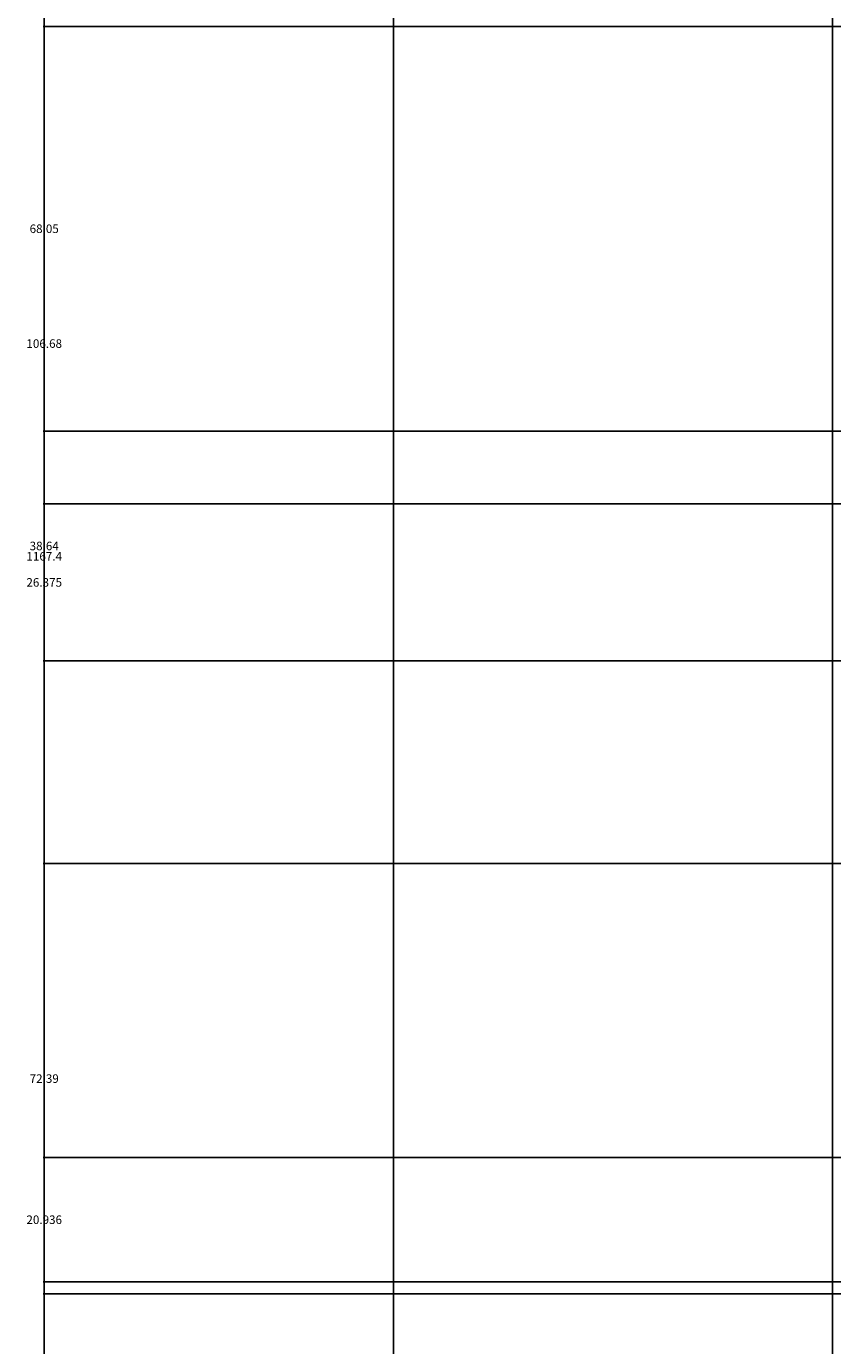
# Model space of a CAD drawing. Units: inches. Extents: x 241 to 943, y 109 to 1396.
# Tile 9 of 34: x 241 to 377, y 620 to 842. Entities that reach past the tile are written whole.
import ezdxf

# ---------------------------------------------------------------- set-up
doc = ezdxf.new("R2010")
doc.units = ezdxf.units.IN
doc.header["$MEASUREMENT"] = 0
doc.layers.add('A-ANNO-DIMS', color=2, linetype='Continuous', lineweight=18)
doc.styles.get("Standard").update_dxf_attribs({"font": 'arial.ttf'})
doc.dimstyles.get("Standard").update_dxf_attribs({"dimtxt": 1.4375, "dimasz": 0.18, "dimexe": 0.18, "dimexo": 0.0625, "dimgap": 0.09, "dimtad": 0, "dimtih": 1, "dimtoh": 1, "dimdec": 4, "dimzin": 0, "dimdsep": 46, "dimlunit": 4, "dimtxsty": 'Standard', "dimcen": 0.09, "dimadec": 0, "dimazin": 0, "dimtfac": 1, "dimtdec": 4, "dimtofl": 0, "dimtmove": 0, "dimatfit": 3, "dimfxl": 1, "dimtolj": 1, "dimtzin": 0, "dimarcsym": 0})

# ---------------------------------------------------------------- blocks, each defined once
blk = doc.blocks.new('*D5')
at = {"layer": 'A-ANNO-DIMS', "color": 0, "lineweight": -2, "transparency": 16777216}
for p, q in [((303.24, 177.8), (303.24, 1395.05)), ((303.42, 1394.87), (338.18, 1394.87)), ((376.86, 1394.87), (342.09, 1394.87)), ((377.04, 177.76), (377.04, 1395.05))]:
    blk.add_line(p, q, dxfattribs=at)
at = {"layer": 'A-ANNO-DIMS', "color": 0, "transparency": 16777216}
for points in [[(303.42, 1394.9), (303.42, 1394.84), (303.24, 1394.87)], [(376.86, 1394.9), (376.86, 1394.84), (377.04, 1394.87)]]:
    blk.add_solid(points, dxfattribs=at)
at = {"layer": 'Defpoints', "color": 0, "transparency": 16777216}
for p in [(377.04, 1394.87), (303.24, 177.74), (377.04, 177.7)]:
    blk.add_point(p, dxfattribs=at)
at = {"layer": 'A-ANNO-DIMS', "color": 0, "transparency": 16777216, "insert": (340.14, 1394.87), "char_height": 1.438, "attachment_point": 5}
blk.add_mtext('\\A1;73.8', dxfattribs=at)
blk = doc.blocks.new('*D7')
at = {"layer": 'A-ANNO-DIMS', "color": 0, "lineweight": -2, "transparency": 16777216}
for p, q in [((508.24, 1336.12), (244.31, 1336.12)), ((244.49, 1335.94), (244.49, 753.25)), ((244.49, 168.92), (244.49, 751.6)), ((303.17, 168.74), (244.31, 168.74))]:
    blk.add_line(p, q, dxfattribs=at)
at = {"layer": 'A-ANNO-DIMS', "color": 0, "transparency": 16777216}
for points in [[(244.46, 1335.94), (244.52, 1335.94), (244.49, 1336.12)], [(244.46, 168.92), (244.52, 168.92), (244.49, 168.74)]]:
    blk.add_solid(points, dxfattribs=at)
at = {"layer": 'Defpoints', "color": 0, "transparency": 16777216}
for p in [(244.49, 1336.12), (508.31, 1336.12), (303.24, 168.74)]:
    blk.add_point(p, dxfattribs=at)
at = {"layer": 'A-ANNO-DIMS', "color": 0, "transparency": 16777216, "insert": (244.49, 752.43), "char_height": 1.438, "attachment_point": 5}
blk.add_mtext('\\A1;1167.4', dxfattribs=at)
blk = doc.blocks.new('*D8')
at = {"layer": 'A-ANNO-DIMS', "color": 0, "lineweight": -2, "transparency": 16777216}
for p, q in [((377.04, 396.94), (377.04, 1395.05)), ((377.22, 1394.87), (380.96, 1394.87)), ((390.71, 1394.87), (386.97, 1394.87)), ((390.89, 384.24), (390.89, 1395.05))]:
    blk.add_line(p, q, dxfattribs=at)
at = {"layer": 'A-ANNO-DIMS', "color": 0, "transparency": 16777216}
for points in [[(377.22, 1394.9), (377.22, 1394.84), (377.04, 1394.87)], [(390.71, 1394.9), (390.71, 1394.84), (390.89, 1394.87)]]:
    blk.add_solid(points, dxfattribs=at)
at = {"layer": 'Defpoints', "color": 0, "transparency": 16777216}
for p in [(390.89, 1394.87), (377.04, 396.88), (390.89, 384.18)]:
    blk.add_point(p, dxfattribs=at)
at = {"layer": 'A-ANNO-DIMS', "color": 0, "transparency": 16777216, "insert": (383.97, 1394.87), "char_height": 1.438, "attachment_point": 5}
blk.add_mtext('\\A1;13.856', dxfattribs=at)
blk = doc.blocks.new('*D21')
at = {"layer": 'A-ANNO-DIMS', "color": 0, "lineweight": -2, "transparency": 16777216}
for p, q in [((376.98, 734.85), (244.31, 734.85)), ((244.49, 734.67), (244.49, 568.67)), ((244.49, 401.01), (244.49, 567.02)), ((376.98, 400.83), (244.31, 400.83))]:
    blk.add_line(p, q, dxfattribs=at)
at = {"layer": 'A-ANNO-DIMS', "color": 0, "transparency": 16777216}
for points in [[(244.46, 734.67), (244.52, 734.67), (244.49, 734.85)], [(244.46, 401.01), (244.52, 401.01), (244.49, 400.83)]]:
    blk.add_solid(points, dxfattribs=at)
at = {"layer": 'Defpoints', "color": 0, "transparency": 16777216}
for p in [(244.49, 734.85), (377.04, 734.85), (377.04, 400.83)]:
    blk.add_point(p, dxfattribs=at)
at = {"layer": 'A-ANNO-DIMS', "color": 0, "transparency": 16777216, "insert": (244.49, 567.84), "char_height": 1.438, "attachment_point": 5}
blk.add_mtext('\\A1;334', dxfattribs=at)
blk = doc.blocks.new('*D22')
at = {"layer": 'A-ANNO-DIMS', "color": 0, "lineweight": -2, "transparency": 16777216}
for p, q in [((376.98, 841.54), (244.31, 841.54)), ((244.49, 841.36), (244.49, 789.02)), ((244.49, 735.03), (244.49, 787.37)), ((376.98, 734.85), (244.31, 734.85))]:
    blk.add_line(p, q, dxfattribs=at)
at = {"layer": 'A-ANNO-DIMS', "color": 0, "transparency": 16777216}
for points in [[(244.46, 841.36), (244.52, 841.36), (244.49, 841.54)], [(244.46, 735.03), (244.52, 735.03), (244.49, 734.85)]]:
    blk.add_solid(points, dxfattribs=at)
at = {"layer": 'Defpoints', "color": 0, "transparency": 16777216}
for p in [(244.49, 841.54), (377.04, 841.54), (377.04, 734.85)]:
    blk.add_point(p, dxfattribs=at)
at = {"layer": 'A-ANNO-DIMS', "color": 0, "transparency": 16777216, "insert": (244.49, 788.2), "char_height": 1.438, "attachment_point": 5}
blk.add_mtext('\\A1;106.68', dxfattribs=at)
blk = doc.blocks.new('*D33')
at = {"layer": 'A-ANNO-DIMS', "color": 0, "lineweight": -2, "transparency": 16777216}
for p, q in [((424.05, 628.4), (244.31, 628.4)), ((244.49, 628.22), (244.49, 599.44)), ((244.49, 569.01), (244.49, 597.79)), ((424.05, 568.83), (244.31, 568.83))]:
    blk.add_line(p, q, dxfattribs=at)
at = {"layer": 'A-ANNO-DIMS', "color": 0, "transparency": 16777216}
for points in [[(244.46, 628.22), (244.52, 628.22), (244.49, 628.4)], [(244.46, 569.01), (244.52, 569.01), (244.49, 568.83)]]:
    blk.add_solid(points, dxfattribs=at)
at = {"layer": 'Defpoints', "color": 0, "transparency": 16777216}
for p in [(244.49, 628.4), (424.11, 628.4), (424.11, 568.83)]:
    blk.add_point(p, dxfattribs=at)
at = {"layer": 'A-ANNO-DIMS', "color": 0, "transparency": 16777216, "insert": (244.49, 598.62), "char_height": 1.438, "attachment_point": 5}
blk.add_mtext('\\A1;59.57', dxfattribs=at)
blk = doc.blocks.new('*D34')
at = {"layer": 'A-ANNO-DIMS', "color": 0, "lineweight": -2, "transparency": 16777216}
for p, q in [((424.05, 700.79), (244.31, 700.79)), ((244.49, 700.61), (244.49, 665.42)), ((244.49, 628.58), (244.49, 663.77)), ((424.05, 628.4), (244.31, 628.4))]:
    blk.add_line(p, q, dxfattribs=at)
at = {"layer": 'A-ANNO-DIMS', "color": 0, "transparency": 16777216}
for points in [[(244.46, 700.61), (244.52, 700.61), (244.49, 700.79)], [(244.46, 628.58), (244.52, 628.58), (244.49, 628.4)]]:
    blk.add_solid(points, dxfattribs=at)
at = {"layer": 'Defpoints', "color": 0, "transparency": 16777216}
for p in [(244.49, 700.79), (424.11, 700.79), (424.11, 628.4)]:
    blk.add_point(p, dxfattribs=at)
at = {"layer": 'A-ANNO-DIMS', "color": 0, "transparency": 16777216, "insert": (244.49, 664.6), "char_height": 1.438, "attachment_point": 5}
blk.add_mtext('\\A1;72.39', dxfattribs=at)
blk = doc.blocks.new('*D35')
at = {"layer": 'A-ANNO-DIMS', "color": 0, "lineweight": -2, "transparency": 16777216}
for p, q in [((388.98, 773.49), (244.31, 773.49)), ((244.49, 773.31), (244.49, 755)), ((244.49, 735.03), (244.49, 753.35)), ((388.98, 734.85), (244.31, 734.85))]:
    blk.add_line(p, q, dxfattribs=at)
at = {"layer": 'A-ANNO-DIMS', "color": 0, "transparency": 16777216}
for points in [[(244.46, 773.31), (244.52, 773.31), (244.49, 773.49)], [(244.46, 735.03), (244.52, 735.03), (244.49, 734.85)]]:
    blk.add_solid(points, dxfattribs=at)
at = {"layer": 'Defpoints', "color": 0, "transparency": 16777216}
for p in [(244.49, 773.49), (389.04, 773.49), (389.04, 734.85)]:
    blk.add_point(p, dxfattribs=at)
at = {"layer": 'A-ANNO-DIMS', "color": 0, "transparency": 16777216, "insert": (244.49, 754.17), "char_height": 1.438, "attachment_point": 5}
blk.add_mtext('\\A1;38.64', dxfattribs=at)
blk = doc.blocks.new('*D36')
at = {"layer": 'A-ANNO-DIMS', "color": 0, "lineweight": -2, "transparency": 16777216}
for p, q in [((396.25, 841.54), (244.31, 841.54)), ((244.49, 841.36), (244.49, 808.34)), ((244.49, 773.67), (244.49, 806.69)), ((396.25, 773.49), (244.31, 773.49))]:
    blk.add_line(p, q, dxfattribs=at)
at = {"layer": 'A-ANNO-DIMS', "color": 0, "transparency": 16777216}
for points in [[(244.46, 841.36), (244.52, 841.36), (244.49, 841.54)], [(244.46, 773.67), (244.52, 773.67), (244.49, 773.49)]]:
    blk.add_solid(points, dxfattribs=at)
at = {"layer": 'Defpoints', "color": 0, "transparency": 16777216}
for p in [(244.49, 841.54), (396.31, 841.54), (396.31, 773.49)]:
    blk.add_point(p, dxfattribs=at)
at = {"layer": 'A-ANNO-DIMS', "color": 0, "transparency": 16777216, "insert": (244.49, 807.51), "char_height": 1.438, "attachment_point": 5}
blk.add_mtext('\\A1;68.05', dxfattribs=at)
blk = doc.blocks.new('*D61')
at = {"layer": 'A-ANNO-DIMS', "color": 0, "lineweight": -2, "transparency": 16777216}
for p, q in [((377.04, 400.89), (377.04, 1395.05)), ((377.22, 1394.87), (398.03, 1394.87)), ((423.93, 1394.87), (403.12, 1394.87)), ((424.11, 568.89), (424.11, 1395.05))]:
    blk.add_line(p, q, dxfattribs=at)
at = {"layer": 'A-ANNO-DIMS', "color": 0, "transparency": 16777216}
for points in [[(377.22, 1394.9), (377.22, 1394.84), (377.04, 1394.87)], [(423.93, 1394.9), (423.93, 1394.84), (424.11, 1394.87)]]:
    blk.add_solid(points, dxfattribs=at)
at = {"layer": 'Defpoints', "color": 0, "transparency": 16777216}
for p in [(424.11, 1394.87), (424.11, 568.83), (377.04, 400.83)]:
    blk.add_point(p, dxfattribs=at)
at = {"layer": 'A-ANNO-DIMS', "color": 0, "transparency": 16777216, "insert": (400.57, 1394.87), "char_height": 1.438, "attachment_point": 5}
blk.add_mtext('\\A1;47.07', dxfattribs=at)
blk = doc.blocks.new('*D91')
at = {"layer": 'A-ANNO-DIMS', "color": 0, "lineweight": -2, "transparency": 16777216}
for p, q in [((377.04, 1070.79), (377.04, 109.81)), ((389.04, 1070.79), (389.04, 109.81)), ((377.22, 109.99), (380.04, 109.99)), ((388.86, 109.99), (386.04, 109.99))]:
    blk.add_line(p, q, dxfattribs=at)
at = {"layer": 'A-ANNO-DIMS', "color": 0, "transparency": 16777216}
for points in [[(377.22, 110.02), (377.22, 109.96), (377.04, 109.99)], [(388.86, 110.02), (388.86, 109.96), (389.04, 109.99)]]:
    blk.add_solid(points, dxfattribs=at)
at = {"layer": 'Defpoints', "color": 0, "transparency": 16777216}
for p in [(377.04, 1070.85), (389.04, 1070.85), (389.04, 109.99)]:
    blk.add_point(p, dxfattribs=at)
at = {"layer": 'A-ANNO-DIMS', "color": 0, "transparency": 16777216, "insert": (383.04, 109.99), "char_height": 1.438, "attachment_point": 5}
blk.add_mtext('\\A1;12.004', dxfattribs=at)
blk = doc.blocks.new('*D131')
at = {"layer": 'A-ANNO-DIMS', "color": 0, "lineweight": -2, "transparency": 16777216}
for p, q in [((446.37, 651.34), (244.31, 651.34)), ((244.49, 651.16), (244.49, 641.69)), ((244.49, 630.58), (244.49, 640.04)), ((446.37, 630.4), (244.31, 630.4))]:
    blk.add_line(p, q, dxfattribs=at)
at = {"layer": 'A-ANNO-DIMS', "color": 0, "transparency": 16777216}
for points in [[(244.46, 651.16), (244.52, 651.16), (244.49, 651.34)], [(244.46, 630.58), (244.52, 630.58), (244.49, 630.4)]]:
    blk.add_solid(points, dxfattribs=at)
at = {"layer": 'Defpoints', "color": 0, "transparency": 16777216}
for p in [(244.49, 651.34), (446.43, 651.34), (446.43, 630.4)]:
    blk.add_point(p, dxfattribs=at)
at = {"layer": 'A-ANNO-DIMS', "color": 0, "transparency": 16777216, "insert": (244.49, 640.87), "char_height": 1.438, "attachment_point": 5}
blk.add_mtext('\\A1;20.936', dxfattribs=at)
blk = doc.blocks.new('*D149')
at = {"layer": 'A-ANNO-DIMS', "color": 0, "lineweight": -2, "transparency": 16777216}
for p, q in [((413.06, 761.23), (244.31, 761.23)), ((244.49, 761.05), (244.49, 748.87)), ((244.49, 735.03), (244.49, 747.22)), ((413.06, 734.85), (244.31, 734.85))]:
    blk.add_line(p, q, dxfattribs=at)
at = {"layer": 'A-ANNO-DIMS', "color": 0, "transparency": 16777216}
for points in [[(244.46, 761.05), (244.52, 761.05), (244.49, 761.23)], [(244.46, 735.03), (244.52, 735.03), (244.49, 734.85)]]:
    blk.add_solid(points, dxfattribs=at)
at = {"layer": 'Defpoints', "color": 0, "transparency": 16777216}
for p in [(244.49, 761.23), (413.12, 761.23), (413.12, 734.85)]:
    blk.add_point(p, dxfattribs=at)
at = {"layer": 'A-ANNO-DIMS', "color": 0, "transparency": 16777216, "insert": (244.49, 748.04), "char_height": 1.438, "attachment_point": 5}
blk.add_mtext('\\A1;26.375', dxfattribs=at)

msp = doc.modelspace()

# ---------------------------------------------------------------- dimensions: what is measured, and where the dimension line sits
at = {"layer": 'A-ANNO-DIMS'}
for base, p1, p2, override, picture, middle in [((377.0391, 1394.8654), (303.2358, 177.7407), (377.0391, 177.6977), {"dimdec": 1, "dimlfac": 1, "dimrnd": 0, "dimzin": 0, "dimdsep": 46, "dimlunit": 2}, '*D5', (340.1375, 1394.8654)), ((390.895, 1394.8654), (377.0391, 396.8782), (390.895, 384.1784), {"dimdec": 3, "dimlfac": 1, "dimrnd": 0, "dimzin": 0, "dimdsep": 46, "dimlunit": 2}, '*D8', (383.9671, 1394.8654)), ((424.1086, 1394.8654), (377.0391, 400.8295), (424.1086, 568.8295), {"dimdec": 2, "dimlfac": 1, "dimrnd": 0, "dimzin": 0, "dimdsep": 46, "dimlunit": 2}, '*D61', (400.5739, 1394.8654)), ((389.0429, 109.9907), (377.0391, 1070.8538), (389.0429, 1070.8538), {"dimdec": 3, "dimlfac": 1, "dimrnd": 0, "dimzin": 0, "dimdsep": 46, "dimlunit": 2}, '*D91', (383.041, 109.9907))]:
    dim = msp.add_linear_dim(base=base, p1=p1, p2=p2, dimstyle='Standard', override=override, dxfattribs=at)
    dim.commit()
    dim.dimension.update_dxf_attribs({"geometry": picture, "text_midpoint": middle})
for base, p1, p2, override, picture, middle in [((244.4858, 1336.1154), (303.2358, 168.7407), (508.3064, 1336.1154), {"dimdec": 1, "dimlfac": 1, "dimrnd": 0, "dimzin": 0, "dimdsep": 46, "dimlunit": 2}, '*D7', (244.4858, 752.4281)), ((244.4858, 841.5382), (377.0391, 734.8538), (377.0391, 841.5382), {"dimdec": 2, "dimlfac": 1, "dimrnd": 0, "dimzin": 0, "dimdsep": 46, "dimlunit": 2}, '*D22', (244.4858, 788.196)), ((244.4858, 841.5382), (396.3125, 773.4916), (396.3125, 841.5382), {"dimdec": 2, "dimlfac": 1, "dimrnd": 0, "dimzin": 0, "dimdsep": 46, "dimlunit": 2}, '*D36', (244.4858, 807.5149)), ((244.4858, 773.4916), (389.0429, 734.8538), (389.0429, 773.4916), {"dimdec": 2, "dimlfac": 1, "dimrnd": 0, "dimzin": 0, "dimdsep": 46, "dimlunit": 2}, '*D35', (244.4858, 754.1727)), ((244.4858, 761.2284), (413.1187, 734.8538), (413.1187, 761.2284), {"dimdec": 3, "dimlfac": 1, "dimrnd": 0, "dimzin": 0, "dimdsep": 46, "dimlunit": 2}, '*D149', (244.4858, 748.0411)), ((244.4858, 734.8538), (377.0391, 400.8295), (377.0391, 734.8538), {"dimdec": 0, "dimlfac": 1, "dimrnd": 0, "dimzin": 0, "dimdsep": 46, "dimlunit": 2}, '*D21', (244.4858, 567.8417)), ((244.4858, 700.7912), (424.1086, 628.4013), (424.1086, 700.7912), {"dimdec": 2, "dimlfac": 1, "dimrnd": 0, "dimzin": 0, "dimdsep": 46, "dimlunit": 2}, '*D34', (244.4858, 664.5962)), ((244.4858, 651.3371), (446.4348, 630.4013), (446.4348, 651.3371), {"dimdec": 3, "dimlfac": 1, "dimrnd": 0, "dimzin": 0, "dimdsep": 46, "dimlunit": 2}, '*D131', (244.4858, 640.8692)), ((244.4858, 628.4013), (424.1086, 568.8295), (424.1086, 628.4013), {"dimdec": 2, "dimlfac": 1, "dimrnd": 0, "dimzin": 0, "dimdsep": 46, "dimlunit": 2}, '*D33', (244.4858, 598.6154))]:
    dim = msp.add_linear_dim(base=base, p1=p1, p2=p2, angle=90, dimstyle='Standard', override=override, dxfattribs=at)
    dim.commit()
    dim.dimension.update_dxf_attribs({"geometry": picture, "text_midpoint": middle})

doc.saveas('drawing.dxf')
